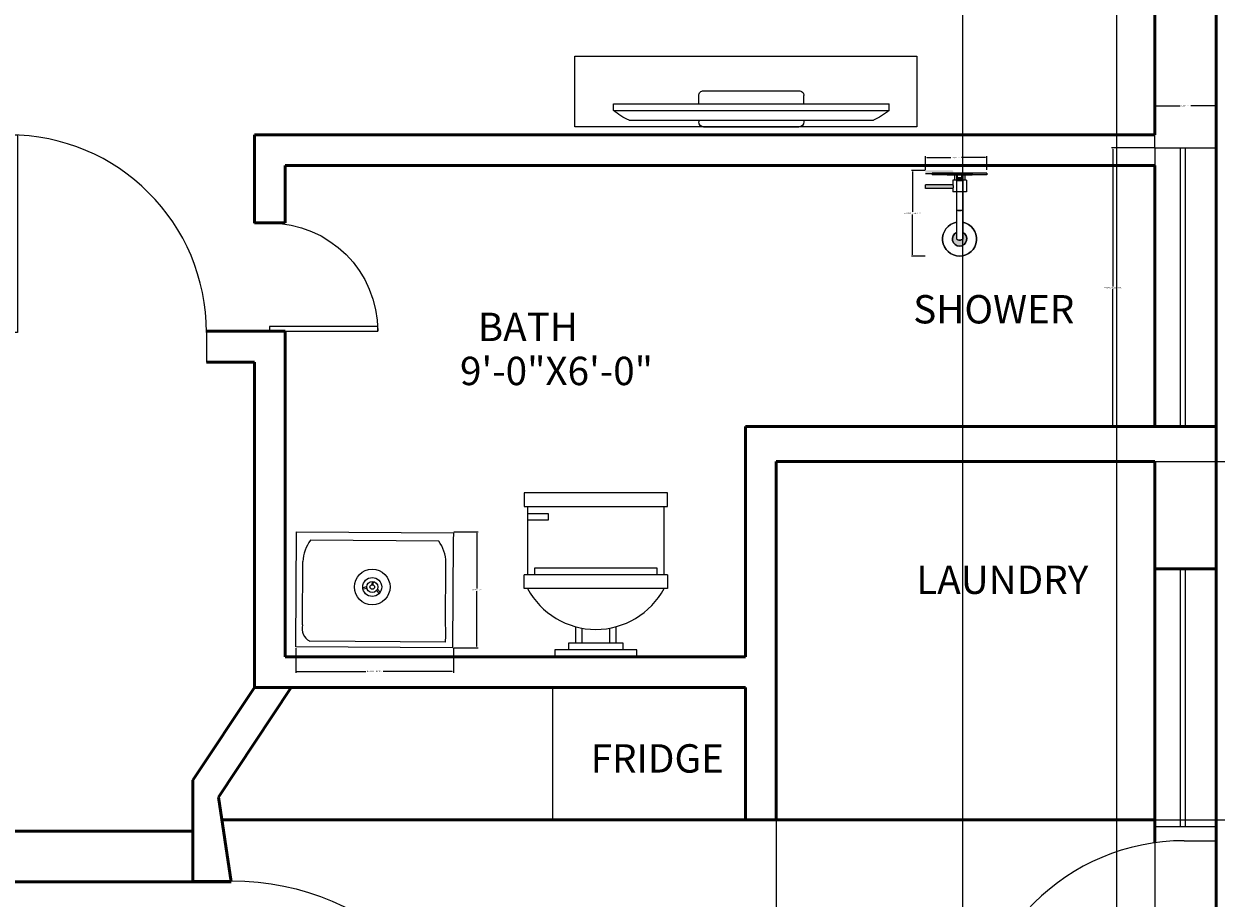
# Model space of a CAD drawing. Units: inches. Extents: x -44 to 461, y -6 to 860.
# Tile 5 of 7: x 184 to 358, y 498 to 626. Entities that reach past the tile are written whole.
import ezdxf

# ---------------------------------------------------------------- set-up
doc = ezdxf.new("R2010")
doc.units = ezdxf.units.IN
doc.header["$MEASUREMENT"] = 0
for name, color, linetype, lineweight in [('A-ANNO-DIMS', 2, 'Continuous', 18), ('A-ANNO-TEXT', 7, 'Continuous', 18), ('A-AREA-IDEN', 7, 'Continuous', 18), ('A-DOOR', 4, 'Continuous', 25), ('A-EQPM', 8, 'Continuous', 18), ('furniture', 30, 'Continuous', 18), ('PLUMBING FIXTURES', 8, 'Continuous', 18), ('walls', 8, 'Continuous', 50), ('windows', 171, 'Continuous', 18)]:
    doc.layers.add(name, color=color, linetype=linetype, lineweight=lineweight)
doc.styles.get("Standard").update_dxf_attribs({"font": 'arial.ttf'})
doc.dimstyles.get("Standard").update_dxf_attribs({"dimtxt": 0.18, "dimasz": 0.18, "dimexe": 0.18, "dimexo": 0.0625, "dimgap": 0.09, "dimtad": 0, "dimtih": 1, "dimtoh": 1, "dimdec": 4, "dimzin": 0, "dimdsep": 46, "dimtxsty": 'Standard', "dimcen": 0.09, "dimadec": 0, "dimazin": 0, "dimtfac": 1, "dimtdec": 4, "dimtofl": 0, "dimtmove": 0, "dimatfit": 3, "dimfxl": 1, "dimtolj": 1, "dimtzin": 0, "dimarcsym": 0})

# ---------------------------------------------------------------- blocks, each defined once
blk = doc.blocks.new('PLASMA-LARGE')
at = {"layer": 'furniture'}
for p, q in [((-7.26, 0), (7.26, 0)), ((-18.61, -1), (18.61, -1)), ((-8, -1), (-8, -0.74)), ((8, -1), (8, -0.74)), ((-21, -2.5), (21, -2.5)), ((-21, -2.5), (-21, -3.5)), ((-21, -3.5), (21, -3.5)), ((-8, -3.5), (-8, -4.76)), ((8, -3.5), (8, -4.76)), ((21, -2.5), (21, -3.5)), ((-7.26, -5.5), (7.26, -5.5))]:
    blk.add_line(p, q, dxfattribs=at)
for centre, radius, start, end in [((-7.26, -0.74), 0.744, 90, 180), ((7.26, -0.74), 0.744, 0, 90), ((-13.97, -11.05), 11.07, 114.7602, 129.4175), ((13.97, -11.05), 11.07, 50.5825, 65.2398), ((-7.26, -4.76), 0.744, 180, 270), ((7.26, -4.76), 0.744, 270, 0)]:
    blk.add_arc(centre, radius, start, end, dxfattribs=at)
blk = doc.blocks.new('*U10')
for p, q in [((-10, 22), (-10, 12)), ((-10, 21), (-7, 21)), ((-7, 21), (-7, 20)), ((10, 12), (10, 22)), ((-7, 20), (-10, 20)), ((9, 13), (-9, 13)), ((-9, 13), (-9, 12)), ((9, 12), (9, 13)), ((10.5, 12), (-10.5, 12)), ((-10.5, 10), (-10.5, 12)), ((10.5, 12), (10.5, 10)), ((10.5, 10), (-10.5, 10)), ((-3, 4.4065), (-3, 2)), ((-2, 2), (-2, 4.1658)), ((2, 4.1658), (2, 2)), ((3, 2), (3, 4.4065)), ((4, 2), (-4, 2)), ((-4, 2), (-4, 1)), ((4, 1), (4, 2))]:
    blk.add_line(p, q)
for points in [[(10.5, 22), (10.5, 24), (-10.5, 24), (-10.5, 22)], [(6, 0), (6, 1), (-6, 1), (-6, 0)]]:
    blk.add_lwpolyline(points, close=True)
blk.add_arc((0, 15.3333), 11.3333, 208.0725, 331.9275)
blk = doc.blocks.new('*U12')
for p, q in [((0, 0), (0, -6)), ((40, 0), (40, -6))]:
    blk.add_line(p, q)
blk.add_lwpolyline([(0, 0), (0, 40), (1.75, 40), (1.75, 0)], close=True)
blk.add_arc((0, 0), 40, 0, 90)
blk = doc.blocks.new('WIN-41IN-FRAME')
for p, q in [((0, 40.98), (9, 40.98)), ((0, 40.98), (0, 0)), ((3.73, 40.98), (3.73, 0)), ((4.5, 0), (4.5, 40.98)), ((9, 40.98), (9, 0)), ((9, 0), (0, 0))]:
    blk.add_line(p, q)
blk = doc.blocks.new('LAV-RECTANGULAR')
for p, q in [((0, 0.15), (0.11, 17)), ((0.11, 17), (23.11, 16.85)), ((20.97, 15.65), (2.16, 15.77)), ((23.11, 16.85), (23.1, 15.71)), ((23.1, 15.71), (23, 0)), ((0.99, 3.35), (1.05, 12.64)), ((21.97, 3.21), (22.03, 12.5)), ((10.4, 8.91), (9.84, 8.81)), ((11.22, 9.73), (11.17, 9.24)), ((11.36, 9.22), (11.4, 9.7)), ((10.52, 8.7), (9.87, 8.58)), ((11.84, 8.39), (12.22, 7.95)), ((11.97, 8.6), (12.36, 8.13)), ((23, 0), (0, 0.15)), ((21.95, 0.84), (2.06, 0.97))]:
    blk.add_line(p, q)
for radius in [2.61, 1.39, 0.816, 0.338]:
    blk.add_circle((11.22, 8.91), radius)
for centre, radius, start, end in [((6.46, 12.5), 5.4, 142.7525, 178.5493), ((16.62, 12.43), 5.4, 0.6949, 36.4918), ((3, 2.82), 2.08, 165.2338, 242.9258), ((12.7, 2.09), 9.33, 352.3124, 6.9318)]:
    blk.add_arc(centre, radius, start, end)
blk = doc.blocks.new('O.H SHOWER-PL')
at = {"layer": 'PLUMBING FIXTURES'}
for points in [[(-1.84, 0), (-1.84, -0.25), (1.84, -0.25), (1.84, 0)], [(0.46, -8.72), (0.46, -9.67, -0.422337), (-0.46, -9.67), (-0.46, -8.72, 4.325472)]]:
    blk.add_hatch(color=256, dxfattribs=at).paths.add_polyline_path(points)
for p, q in [((-1.84, 0), (-1.84, -0.25)), ((1.84, 0), (-1.84, 0)), ((1.84, 0), (1.84, -0.25)), ((1.84, -0.25), (-1.84, -0.25)), ((-0.46, -0.25), (-0.46, -9.67)), ((0.46, -0.25), (0.46, -9.67))]:
    blk.add_line(p, q, dxfattribs=at)
for centre, radius, start, end in [((0, -4.48), 1.03, 243.53, 296.47), ((0, -9.67), 2.5, 100.61, 79.39), ((0, -9.67), 1.05, 116.0349, 63.9652), ((0, -9.22), 0.643, 224.2078, 315.7922)]:
    blk.add_arc(centre, radius, start, end, dxfattribs=at)
blk = doc.blocks.new('DIVERTER-PL')
at = {"layer": 'PLUMBING FIXTURES'}
for points in [[(4, 0), (-4, 0), (-4, -0.25), (4, -0.25)], [(0.38, -1.14), (0.38, -0.7), (-0.37, -0.7), (-0.37, -1.14)], [(1, -1.75, 0.30818), (1, -2.25), (5, -2.25), (5, -1.75)]]:
    blk.add_hatch(color=256, dxfattribs=at).paths.add_polyline_path(points)
for p, q in [((-4, 0), (-4, -0.25)), ((-4, 0), (4, 0)), ((4, 0), (4, -0.25)), ((-4, -0.25), (4, -0.25)), ((-4, -0.25), (4, -0.25)), ((-1, -1.05), (-0.37, -1.05)), ((-1, -1.05), (-1, -2.75)), ((-0.75, -0.25), (-0.75, -1.05)), ((-0.37, -0.7), (0.38, -0.7)), ((-0.37, -0.7), (-0.37, -1.14)), ((-0.37, -1.14), (0.38, -1.14)), ((-0.32, -0.7), (-0.32, -0.25)), ((0.32, -0.7), (0.32, -0.25)), ((0.38, -0.7), (0.38, -1.14)), ((0.38, -1.05), (1, -1.05)), ((0.75, -0.25), (0.75, -1.05)), ((1, -1.05), (1, -1.75)), ((-1, -2.75), (1, -2.75)), ((1, -2.25), (1, -2.75))]:
    blk.add_line(p, q, dxfattribs=at)
at = {"layer": 'PLUMBING FIXTURES', "ltscale": 12}
for p, q in [((1, -1.75), (5, -1.75)), ((1, -2.25), (5, -2.25)), ((5, -2.25), (5, -1.75))]:
    blk.add_line(p, q, dxfattribs=at)
at = {"layer": 'PLUMBING FIXTURES'}
blk.add_arc((1.37, -2), 0.444, 145.7435, 214.2565, dxfattribs=at)
blk = doc.blocks.new('A$C7F153053')
at = {"layer": 'PLUMBING FIXTURES', "xscale": -1, "rotation": 270}
for name in ['DIVERTER-PL', 'O.H SHOWER-PL']:
    blk.add_blockref(name, (12.17, 4), dxfattribs=at)
blk = doc.blocks.new('SHOWER-HEAD-AND-DIVERTER')
for points in [[(4, 12.56, -0.30818), (4, 12.06), (0, 12.06), (0, 12.56)], [(4, 12.56, -0.30818), (4, 12.06), (0, 12.06), (0, 12.56)], [(4, 12.56, -0.30818), (4, 12.06), (0, 12.06), (0, 12.56)], [(4, 12.56, -0.30818), (4, 12.06), (0, 12.06), (0, 12.56)], [(4, 12.56, -0.30818), (4, 12.06), (0, 12.06), (0, 12.56)], [(4, 12.56, -0.30818), (4, 12.06), (0, 12.06), (0, 12.56)], [(4, 12.56, -0.30818), (4, 12.06), (0, 12.06), (0, 12.56)], [(4, 12.56, -0.30818), (4, 12.06), (0, 12.06), (0, 12.56)], [(4, 12.56, -0.30818), (4, 12.06), (0, 12.06), (0, 12.56)], [(4, 12.56, -0.30818), (4, 12.06), (0, 12.06), (0, 12.56)], [(4, 12.56, -0.30818), (4, 12.06), (0, 12.06), (0, 12.56)], [(4, 12.56, -0.30818), (4, 12.06), (0, 12.06), (0, 12.56)], [(4, 12.56, -0.30818), (4, 12.06), (0, 12.06), (0, 12.56)], [(4, 12.56, -0.30818), (4, 12.06), (0, 12.06), (0, 12.56)], [(4, 12.56, -0.30818), (4, 12.06), (0, 12.06), (0, 12.56)], [(4, 12.56, -0.30818), (4, 12.06), (0, 12.06), (0, 12.56)], [(4, 12.56, -0.30818), (4, 12.06), (0, 12.06), (0, 12.56)], [(4, 12.56, -0.30818), (4, 12.06), (0, 12.06), (0, 12.56)], [(4, 12.56, -0.30818), (4, 12.06), (0, 12.06), (0, 12.56)], [(4, 12.56, -0.30818), (4, 12.06), (0, 12.06), (0, 12.56)], [(4, 12.56, -0.30818), (4, 12.06), (0, 12.06), (0, 12.56)], [(4, 12.56, -0.30818), (4, 12.06), (0, 12.06), (0, 12.56)], [(4, 12.56, -0.30818), (4, 12.06), (0, 12.06), (0, 12.56)], [(4, 12.56, -0.30818), (4, 12.06), (0, 12.06), (0, 12.56)], [(4, 12.56, -0.30818), (4, 12.06), (0, 12.06), (0, 12.56)], [(4, 12.56, -0.30818), (4, 12.06), (0, 12.06), (0, 12.56)], [(4, 12.56, -0.30818), (4, 12.06), (0, 12.06), (0, 12.56)], [(4, 12.56, -0.30818), (4, 12.06), (0, 12.06), (0, 12.56)], [(4, 12.56, -0.30818), (4, 12.06), (0, 12.06), (0, 12.56)], [(4, 12.56, -0.30818), (4, 12.06), (0, 12.06), (0, 12.56)], [(4, 12.56, -0.30818), (4, 12.06), (0, 12.06), (0, 12.56)], [(4, 12.56, -0.30818), (4, 12.06), (0, 12.06), (0, 12.56)], [(4, 12.56, -0.30818), (4, 12.06), (0, 12.06), (0, 12.56)], [(4, 12.56, -0.30818), (4, 12.06), (0, 12.06), (0, 12.56)], [(4, 12.56, -0.30818), (4, 12.06), (0, 12.06), (0, 12.56)], [(4, 12.56, -0.30818), (4, 12.06), (0, 12.06), (0, 12.56)], [(4.54, 3.44), (4.54, 2.5, 0.422337), (5.46, 2.5), (5.46, 3.44, -4.325472)], [(4.54, 3.44), (4.54, 2.5, 0.422337), (5.46, 2.5), (5.46, 3.44, -4.325472)], [(4.54, 3.44), (4.54, 2.5, 0.422337), (5.46, 2.5), (5.46, 3.44, -4.325472)], [(4.54, 3.44), (4.54, 2.5, 0.422337), (5.46, 2.5), (5.46, 3.44, -4.325472)], [(4.54, 3.44), (4.54, 2.5, 0.422337), (5.46, 2.5), (5.46, 3.44, -4.325472)], [(4.54, 3.44), (4.54, 2.5, 0.422337), (5.46, 2.5), (5.46, 3.44, -4.325472)], [(4.54, 3.44), (4.54, 2.5, 0.422337), (5.46, 2.5), (5.46, 3.44, -4.325472)], [(4.54, 3.44), (4.54, 2.5, 0.422337), (5.46, 2.5), (5.46, 3.44, -4.325472)], [(4.54, 3.44), (4.54, 2.5, 0.422337), (5.46, 2.5), (5.46, 3.44, -4.325472)], [(4.54, 3.44), (4.54, 2.5, 0.422337), (5.46, 2.5), (5.46, 3.44, -4.325472)], [(4.54, 3.44), (4.54, 2.5, 0.422337), (5.46, 2.5), (5.46, 3.44, -4.325472)], [(4.54, 3.44), (4.54, 2.5, 0.422337), (5.46, 2.5), (5.46, 3.44, -4.325472)], [(4.54, 3.44), (4.54, 2.5, 0.422337), (5.46, 2.5), (5.46, 3.44, -4.325472)], [(4.54, 3.44), (4.54, 2.5, 0.422337), (5.46, 2.5), (5.46, 3.44, -4.325472)], [(4.54, 3.44), (4.54, 2.5, 0.422337), (5.46, 2.5), (5.46, 3.44, -4.325472)], [(4.54, 3.44), (4.54, 2.5, 0.422337), (5.46, 2.5), (5.46, 3.44, -4.325472)], [(4.54, 3.44), (4.54, 2.5, 0.422337), (5.46, 2.5), (5.46, 3.44, -4.325472)], [(4.54, 3.44), (4.54, 2.5, 0.422337), (5.46, 2.5), (5.46, 3.44, -4.325472)], [(4.54, 3.44), (4.54, 2.5, 0.422337), (5.46, 2.5), (5.46, 3.44, -4.325472)], [(4.54, 3.44), (4.54, 2.5, 0.422337), (5.46, 2.5), (5.46, 3.44, -4.325472)], [(4.54, 3.44), (4.54, 2.5, 0.422337), (5.46, 2.5), (5.46, 3.44, -4.325472)], [(4.54, 3.44), (4.54, 2.5, 0.422337), (5.46, 2.5), (5.46, 3.44, -4.325472)], [(4.54, 3.44), (4.54, 2.5, 0.422337), (5.46, 2.5), (5.46, 3.44, -4.325472)], [(4.54, 3.44), (4.54, 2.5, 0.422337), (5.46, 2.5), (5.46, 3.44, -4.325472)], [(4.54, 3.44), (4.54, 2.5, 0.422337), (5.46, 2.5), (5.46, 3.44, -4.325472)], [(4.54, 3.44), (4.54, 2.5, 0.422337), (5.46, 2.5), (5.46, 3.44, -4.325472)], [(4.54, 3.44), (4.54, 2.5, 0.422337), (5.46, 2.5), (5.46, 3.44, -4.325472)], [(4.54, 3.44), (4.54, 2.5, 0.422337), (5.46, 2.5), (5.46, 3.44, -4.325472)], [(4.54, 3.44), (4.54, 2.5, 0.422337), (5.46, 2.5), (5.46, 3.44, -4.325472)], [(4.54, 3.44), (4.54, 2.5, 0.422337), (5.46, 2.5), (5.46, 3.44, -4.325472)], [(4.54, 3.44), (4.54, 2.5, 0.422337), (5.46, 2.5), (5.46, 3.44, -4.325472)], [(4.54, 3.44), (4.54, 2.5, 0.422337), (5.46, 2.5), (5.46, 3.44, -4.325472)], [(4.54, 3.44), (4.54, 2.5, 0.422337), (5.46, 2.5), (5.46, 3.44, -4.325472)], [(4.54, 3.44), (4.54, 2.5, 0.422337), (5.46, 2.5), (5.46, 3.44, -4.325472)], [(4.54, 3.44), (4.54, 2.5, 0.422337), (5.46, 2.5), (5.46, 3.44, -4.325472)], [(4.54, 3.44), (4.54, 2.5, 0.422337), (5.46, 2.5), (5.46, 3.44, -4.325472)], [(4.54, 3.44), (4.54, 2.5, 0.422337), (5.46, 2.5), (5.46, 3.44, -4.325472)], [(4.54, 3.44), (4.54, 2.5, 0.422337), (5.46, 2.5), (5.46, 3.44, -4.325472)]]:
    blk.add_hatch(color=256).paths.add_polyline_path(points)
at = {"ltscale": 12}
blk.add_line((4, 12.06), (0, 12.06), dxfattribs=at)
blk.add_line((4, 12.06), (0, 12.06), dxfattribs=at)
blk.add_line((4, 12.06), (0, 12.06), dxfattribs=at)
blk.add_line((4, 12.06), (0, 12.06), dxfattribs=at)
blk.add_line((4, 12.06), (0, 12.06), dxfattribs=at)
blk.add_line((4, 12.06), (0, 12.06), dxfattribs=at)
blk.add_line((4, 12.06), (0, 12.06), dxfattribs=at)
blk.add_line((4, 12.06), (0, 12.06), dxfattribs=at)
blk.add_line((4, 12.06), (0, 12.06), dxfattribs=at)
blk.add_line((4, 12.06), (0, 12.06), dxfattribs=at)
blk.add_line((4, 12.06), (0, 12.06), dxfattribs=at)
blk.add_line((4, 12.06), (0, 12.06), dxfattribs=at)
blk.add_line((4, 12.06), (0, 12.06), dxfattribs=at)
blk.add_line((4, 12.06), (0, 12.06), dxfattribs=at)
blk.add_line((4, 12.06), (0, 12.06), dxfattribs=at)
blk.add_line((4, 12.06), (0, 12.06), dxfattribs=at)
blk.add_line((4, 12.06), (0, 12.06), dxfattribs=at)
blk.add_line((4, 12.06), (0, 12.06), dxfattribs=at)
blk.add_line((4, 12.06), (0, 12.06), dxfattribs=at)
blk.add_line((4, 12.06), (0, 12.06), dxfattribs=at)
blk.add_line((4, 12.06), (0, 12.06), dxfattribs=at)
blk.add_line((4, 12.06), (0, 12.06), dxfattribs=at)
blk.add_line((4, 12.06), (0, 12.06), dxfattribs=at)
blk.add_line((4, 12.06), (0, 12.06), dxfattribs=at)
blk.add_line((4, 12.06), (0, 12.06), dxfattribs=at)
blk.add_line((4, 12.06), (0, 12.06), dxfattribs=at)
blk.add_line((4, 12.06), (0, 12.06), dxfattribs=at)
blk.add_line((4, 12.06), (0, 12.06), dxfattribs=at)
blk.add_line((4, 12.06), (0, 12.06), dxfattribs=at)
blk.add_line((4, 12.06), (0, 12.06), dxfattribs=at)
blk.add_line((4, 12.06), (0, 12.06), dxfattribs=at)
blk.add_line((4, 12.06), (0, 12.06), dxfattribs=at)
blk.add_line((4, 12.06), (0, 12.06), dxfattribs=at)
blk.add_line((4, 12.06), (0, 12.06), dxfattribs=at)
blk.add_line((4, 12.06), (0, 12.06), dxfattribs=at)
blk.add_line((4, 12.06), (0, 12.06), dxfattribs=at)
blk.add_line((4, 12.06), (0, 12.06), dxfattribs=at)
blk.add_line((4, 12.06), (0, 12.06), dxfattribs=at)
for p, q in [((4.54, 11.92), (4.54, 2.5)), ((4.54, 11.92), (4.54, 2.5)), ((4.54, 11.92), (4.54, 2.5)), ((4.54, 11.92), (4.54, 2.5)), ((4.54, 11.92), (4.54, 2.5)), ((4.54, 11.92), (4.54, 2.5)), ((4.54, 11.92), (4.54, 2.5)), ((4.54, 11.92), (4.54, 2.5)), ((4.54, 11.92), (4.54, 2.5)), ((4.54, 11.92), (4.54, 2.5)), ((4.54, 11.92), (4.54, 2.5)), ((4.54, 11.92), (4.54, 2.5)), ((4.54, 11.92), (4.54, 2.5)), ((4.54, 11.92), (4.54, 2.5)), ((4.54, 11.92), (4.54, 2.5)), ((4.54, 11.92), (4.54, 2.5)), ((4.54, 11.92), (4.54, 2.5)), ((4.54, 11.92), (4.54, 2.5)), ((4.54, 11.92), (4.54, 2.5)), ((4.54, 11.92), (4.54, 2.5)), ((4.54, 11.92), (4.54, 2.5)), ((4.54, 11.92), (4.54, 2.5)), ((4.54, 11.92), (4.54, 2.5)), ((4.54, 11.92), (4.54, 2.5)), ((4.54, 11.92), (4.54, 2.5)), ((4.54, 11.92), (4.54, 2.5)), ((4.54, 11.92), (4.54, 2.5)), ((4.54, 11.92), (4.54, 2.5)), ((4.54, 11.92), (4.54, 2.5)), ((4.54, 11.92), (4.54, 2.5)), ((4.54, 11.92), (4.54, 2.5)), ((4.54, 11.92), (4.54, 2.5)), ((4.54, 11.92), (4.54, 2.5)), ((4.54, 11.92), (4.54, 2.5)), ((4.54, 11.92), (4.54, 2.5)), ((4.54, 11.92), (4.54, 2.5)), ((4.54, 11.92), (4.54, 2.5)), ((4.54, 11.92), (4.54, 2.5)), ((5.46, 11.92), (5.46, 2.5)), ((5.46, 11.92), (5.46, 2.5)), ((5.46, 11.92), (5.46, 2.5)), ((5.46, 11.92), (5.46, 2.5)), ((5.46, 11.92), (5.46, 2.5)), ((5.46, 11.92), (5.46, 2.5)), ((5.46, 11.92), (5.46, 2.5)), ((5.46, 11.92), (5.46, 2.5)), ((5.46, 11.92), (5.46, 2.5)), ((5.46, 11.92), (5.46, 2.5)), ((5.46, 11.92), (5.46, 2.5)), ((5.46, 11.92), (5.46, 2.5)), ((5.46, 11.92), (5.46, 2.5)), ((5.46, 11.92), (5.46, 2.5)), ((5.46, 11.92), (5.46, 2.5)), ((5.46, 11.92), (5.46, 2.5)), ((5.46, 11.92), (5.46, 2.5)), ((5.46, 11.92), (5.46, 2.5)), ((5.46, 11.92), (5.46, 2.5)), ((5.46, 11.92), (5.46, 2.5)), ((5.46, 11.92), (5.46, 2.5)), ((5.46, 11.92), (5.46, 2.5)), ((5.46, 11.92), (5.46, 2.5)), ((5.46, 11.92), (5.46, 2.5)), ((5.46, 11.92), (5.46, 2.5)), ((5.46, 11.92), (5.46, 2.5)), ((5.46, 11.92), (5.46, 2.5)), ((5.46, 11.92), (5.46, 2.5)), ((5.46, 11.92), (5.46, 2.5)), ((5.46, 11.92), (5.46, 2.5)), ((5.46, 11.92), (5.46, 2.5)), ((5.46, 11.92), (5.46, 2.5)), ((5.46, 11.92), (5.46, 2.5)), ((5.46, 11.92), (5.46, 2.5)), ((5.46, 11.92), (5.46, 2.5)), ((5.46, 11.92), (5.46, 2.5)), ((5.46, 11.92), (5.46, 2.5)), ((5.46, 11.92), (5.46, 2.5))]:
    blk.add_line(p, q)
for centre, radius, start, end in [((5, 7.69), 1.03, 243.53, 296.47), ((5, 7.69), 1.03, 243.53, 296.47), ((5, 7.69), 1.03, 243.53, 296.47), ((5, 7.69), 1.03, 243.53, 296.47), ((5, 7.69), 1.03, 243.53, 296.47), ((5, 7.69), 1.03, 243.53, 296.47), ((5, 7.69), 1.03, 243.53, 296.47), ((5, 7.69), 1.03, 243.53, 296.47), ((5, 7.69), 1.03, 243.53, 296.47), ((5, 7.69), 1.03, 243.53, 296.47), ((5, 7.69), 1.03, 243.53, 296.47), ((5, 7.69), 1.03, 243.53, 296.47), ((5, 7.69), 1.03, 243.53, 296.47), ((5, 7.69), 1.03, 243.53, 296.47), ((5, 7.69), 1.03, 243.53, 296.47), ((5, 7.69), 1.03, 243.53, 296.47), ((5, 7.69), 1.03, 243.53, 296.47), ((5, 7.69), 1.03, 243.53, 296.47), ((5, 7.69), 1.03, 243.53, 296.47), ((5, 7.69), 1.03, 243.53, 296.47), ((5, 7.69), 1.03, 243.53, 296.47), ((5, 7.69), 1.03, 243.53, 296.47), ((5, 7.69), 1.03, 243.53, 296.47), ((5, 7.69), 1.03, 243.53, 296.47), ((5, 7.69), 1.03, 243.53, 296.47), ((5, 7.69), 1.03, 243.53, 296.47), ((5, 7.69), 1.03, 243.53, 296.47), ((5, 7.69), 1.03, 243.53, 296.47), ((5, 7.69), 1.03, 243.53, 296.47), ((5, 7.69), 1.03, 243.53, 296.47), ((5, 7.69), 1.03, 243.53, 296.47), ((5, 7.69), 1.03, 243.53, 296.47), ((5, 7.69), 1.03, 243.53, 296.47), ((5, 7.69), 1.03, 243.53, 296.47), ((5, 7.69), 1.03, 243.53, 296.47), ((5, 7.69), 1.03, 243.53, 296.47), ((5, 7.69), 1.03, 243.53, 296.47), ((5, 7.69), 1.03, 243.53, 296.47), ((5, 2.5), 2.5, 100.61, 79.39), ((5, 2.5), 2.5, 100.61, 79.39), ((5, 2.5), 2.5, 100.61, 79.39), ((5, 2.5), 2.5, 100.61, 79.39), ((5, 2.5), 2.5, 100.61, 79.39), ((5, 2.5), 2.5, 100.61, 79.39), ((5, 2.5), 2.5, 100.61, 79.39), ((5, 2.5), 2.5, 100.61, 79.39), ((5, 2.5), 2.5, 100.61, 79.39), ((5, 2.5), 2.5, 100.61, 79.39), ((5, 2.5), 2.5, 100.61, 79.39), ((5, 2.5), 2.5, 100.61, 79.39), ((5, 2.5), 2.5, 100.61, 79.39), ((5, 2.5), 2.5, 100.61, 79.39), ((5, 2.5), 2.5, 100.61, 79.39), ((5, 2.5), 2.5, 100.61, 79.39), ((5, 2.5), 2.5, 100.61, 79.39), ((5, 2.5), 2.5, 100.61, 79.39), ((5, 2.5), 2.5, 100.61, 79.39), ((5, 2.5), 2.5, 100.61, 79.39), ((5, 2.5), 2.5, 100.61, 79.39), ((5, 2.5), 2.5, 100.61, 79.39), ((5, 2.5), 2.5, 100.61, 79.39), ((5, 2.5), 2.5, 100.61, 79.39), ((5, 2.5), 2.5, 100.61, 79.39), ((5, 2.5), 2.5, 100.61, 79.39), ((5, 2.5), 2.5, 100.61, 79.39), ((5, 2.5), 2.5, 100.61, 79.39), ((5, 2.5), 2.5, 100.61, 79.39), ((5, 2.5), 2.5, 100.61, 79.39), ((5, 2.5), 2.5, 100.61, 79.39), ((5, 2.5), 2.5, 100.61, 79.39), ((5, 2.5), 2.5, 100.61, 79.39), ((5, 2.5), 2.5, 100.61, 79.39), ((5, 2.5), 2.5, 100.61, 79.39), ((5, 2.5), 2.5, 100.61, 79.39), ((5, 2.5), 2.5, 100.61, 79.39), ((5, 2.5), 2.5, 100.61, 79.39), ((5, 2.5), 1.05, 116.0348, 63.9651), ((5, 2.5), 1.05, 116.0348, 63.9651), ((5, 2.5), 1.05, 116.0348, 63.9651), ((5, 2.5), 1.05, 116.0348, 63.9651), ((5, 2.5), 1.05, 116.0348, 63.9651), ((5, 2.5), 1.05, 116.0348, 63.9651), ((5, 2.5), 1.05, 116.0348, 63.9651), ((5, 2.5), 1.05, 116.0348, 63.9651), ((5, 2.5), 1.05, 116.0348, 63.9651), ((5, 2.5), 1.05, 116.0348, 63.9651), ((5, 2.5), 1.05, 116.0348, 63.9651), ((5, 2.5), 1.05, 116.0348, 63.9651), ((5, 2.5), 1.05, 116.0348, 63.9651), ((5, 2.5), 1.05, 116.0348, 63.9651), ((5, 2.5), 1.05, 116.0348, 63.9651), ((5, 2.5), 1.05, 116.0348, 63.9651), ((5, 2.5), 1.05, 116.0348, 63.9651), ((5, 2.5), 1.05, 116.0348, 63.9651), ((5, 2.5), 1.05, 116.0348, 63.9651), ((5, 2.5), 1.05, 116.0348, 63.9651), ((5, 2.5), 1.05, 116.0348, 63.9651), ((5, 2.5), 1.05, 116.0348, 63.9651), ((5, 2.5), 1.05, 116.0348, 63.9651), ((5, 2.5), 1.05, 116.0348, 63.9651), ((5, 2.5), 1.05, 116.0348, 63.9651), ((5, 2.5), 1.05, 116.0348, 63.9651), ((5, 2.5), 1.05, 116.0348, 63.9651), ((5, 2.5), 1.05, 116.0348, 63.9651), ((5, 2.5), 1.05, 116.0348, 63.9651), ((5, 2.5), 1.05, 116.0348, 63.9651), ((5, 2.5), 1.05, 116.0348, 63.9651), ((5, 2.5), 1.05, 116.0348, 63.9651), ((5, 2.5), 1.05, 116.0348, 63.9651), ((5, 2.5), 1.05, 116.0348, 63.9651), ((5, 2.5), 1.05, 116.0348, 63.9651), ((5, 2.5), 1.05, 116.0348, 63.9651), ((5, 2.5), 1.05, 116.0348, 63.9651), ((5, 2.5), 1.05, 116.0348, 63.9651), ((5, 2.95), 0.643, 224.2078, 315.7922), ((5, 2.95), 0.643, 224.2078, 315.7922), ((5, 2.95), 0.643, 224.2078, 315.7922), ((5, 2.95), 0.643, 224.2078, 315.7922), ((5, 2.95), 0.643, 224.2078, 315.7922), ((5, 2.95), 0.643, 224.2078, 315.7922), ((5, 2.95), 0.643, 224.2078, 315.7922), ((5, 2.95), 0.643, 224.2078, 315.7922), ((5, 2.95), 0.643, 224.2078, 315.7922), ((5, 2.95), 0.643, 224.2078, 315.7922), ((5, 2.95), 0.643, 224.2078, 315.7922), ((5, 2.95), 0.643, 224.2078, 315.7922), ((5, 2.95), 0.643, 224.2078, 315.7922), ((5, 2.95), 0.643, 224.2078, 315.7922), ((5, 2.95), 0.643, 224.2078, 315.7922), ((5, 2.95), 0.643, 224.2078, 315.7922), ((5, 2.95), 0.643, 224.2078, 315.7922), ((5, 2.95), 0.643, 224.2078, 315.7922), ((5, 2.95), 0.643, 224.2078, 315.7922), ((5, 2.95), 0.643, 224.2078, 315.7922), ((5, 2.95), 0.643, 224.2078, 315.7922), ((5, 2.95), 0.643, 224.2078, 315.7922), ((5, 2.95), 0.643, 224.2078, 315.7922), ((5, 2.95), 0.643, 224.2078, 315.7922), ((5, 2.95), 0.643, 224.2078, 315.7922), ((5, 2.95), 0.643, 224.2078, 315.7922), ((5, 2.95), 0.643, 224.2078, 315.7922), ((5, 2.95), 0.643, 224.2078, 315.7922), ((5, 2.95), 0.643, 224.2078, 315.7922), ((5, 2.95), 0.643, 224.2078, 315.7922), ((5, 2.95), 0.643, 224.2078, 315.7922), ((5, 2.95), 0.643, 224.2078, 315.7922), ((5, 2.95), 0.643, 224.2078, 315.7922), ((5, 2.95), 0.643, 224.2078, 315.7922), ((5, 2.95), 0.643, 224.2078, 315.7922), ((5, 2.95), 0.643, 224.2078, 315.7922), ((5, 2.95), 0.643, 224.2078, 315.7922), ((5, 2.95), 0.643, 224.2078, 315.7922)]:
    blk.add_arc(centre, radius, start, end)
at = {"ltscale": 35, "rotation": 89.99999999999999}
blk.add_blockref('A$C7F153053', (9, 0), dxfattribs=at)
blk = doc.blocks.new('*D26')
at = {"layer": 'A-ANNO-DIMS', "color": 0, "lineweight": -2, "transparency": 16777216}
for p, q in [((349.38, 608.14), (343.12, 608.14)), ((343.3, 607.96), (343.3, 587.83)), ((343.3, 567.34), (343.3, 587.47)), ((349.38, 567.16), (343.12, 567.16))]:
    blk.add_line(p, q, dxfattribs=at)
at = {"layer": 'A-ANNO-DIMS', "color": 0, "transparency": 16777216}
for points in [[(343.27, 607.96), (343.33, 607.96), (343.3, 608.14)], [(343.27, 567.34), (343.33, 567.34), (343.3, 567.16)]]:
    blk.add_solid(points, dxfattribs=at)
at = {"layer": 'Defpoints', "color": 0, "transparency": 16777216}
for p in [(343.3, 608.14), (349.45, 608.14), (349.45, 567.16)]:
    blk.add_point(p, dxfattribs=at)
at = {"layer": 'A-ANNO-DIMS', "color": 0, "transparency": 16777216, "insert": (343.3, 587.65), "char_height": 0.18, "attachment_point": 5}
blk.add_mtext('\\A1;WINDOW 40.9847 TYP.', dxfattribs=at)
blk = doc.blocks.new('*D27')
at = {"layer": 'A-ANNO-DIMS', "color": 0, "lineweight": -2, "transparency": 16777216}
for p, q in [((349.45, 608.21), (349.45, 614.47)), ((349.63, 614.29), (353.17, 614.29)), ((358.27, 614.29), (354.72, 614.29)), ((358.45, 608.21), (358.45, 614.47))]:
    blk.add_line(p, q, dxfattribs=at)
at = {"layer": 'A-ANNO-DIMS', "color": 0, "transparency": 16777216}
for points in [[(349.63, 614.32), (349.63, 614.26), (349.45, 614.29)], [(358.27, 614.32), (358.27, 614.26), (358.45, 614.29)]]:
    blk.add_solid(points, dxfattribs=at)
at = {"layer": 'Defpoints', "color": 0, "transparency": 16777216}
for p in [(358.45, 614.29), (349.45, 608.14), (358.45, 608.14)]:
    blk.add_point(p, dxfattribs=at)
at = {"layer": 'A-ANNO-DIMS', "color": 0, "transparency": 16777216, "insert": (353.95, 614.29), "char_height": 0.18, "attachment_point": 5}
blk.add_mtext('\\A1;9.0000 TYP.', dxfattribs=at)
blk = doc.blocks.new('*D42')
at = {"layer": 'A-ANNO-DIMS', "color": 0, "lineweight": -2, "transparency": 16777216}
for p, q in [((223.5, 534.8), (223.5, 531.21)), ((246.61, 534.8), (246.61, 531.21)), ((223.68, 531.39), (233.8, 531.39)), ((246.43, 531.39), (236.3, 531.39))]:
    blk.add_line(p, q, dxfattribs=at)
at = {"layer": 'A-ANNO-DIMS', "color": 0, "transparency": 16777216}
for points in [[(223.68, 531.42), (223.68, 531.36), (223.5, 531.39)], [(246.43, 531.42), (246.43, 531.36), (246.61, 531.39)]]:
    blk.add_solid(points, dxfattribs=at)
at = {"layer": 'Defpoints', "color": 0, "transparency": 16777216}
for p in [(223.5, 534.86), (246.61, 534.86), (246.61, 531.39)]:
    blk.add_point(p, dxfattribs=at)
at = {"layer": 'A-ANNO-DIMS', "color": 0, "transparency": 16777216, "insert": (235.05, 531.39), "char_height": 0.18, "attachment_point": 5}
blk.add_mtext('\\A1;BASIN 23.1070 TYP.', dxfattribs=at)
blk = doc.blocks.new('*D43')
at = {"layer": 'A-ANNO-DIMS', "color": 0, "lineweight": -2, "transparency": 16777216}
for p, q in [((246.67, 551.86), (250.25, 551.86)), ((250.07, 551.68), (250.07, 543.54)), ((250.07, 535.04), (250.07, 543.18)), ((246.67, 534.86), (250.25, 534.86))]:
    blk.add_line(p, q, dxfattribs=at)
at = {"layer": 'A-ANNO-DIMS', "color": 0, "transparency": 16777216}
for points in [[(250.04, 551.68), (250.1, 551.68), (250.07, 551.86)], [(250.04, 535.04), (250.1, 535.04), (250.07, 534.86)]]:
    blk.add_solid(points, dxfattribs=at)
at = {"layer": 'Defpoints', "color": 0, "transparency": 16777216}
for p in [(246.61, 551.86), (250.07, 551.86), (246.61, 534.86)]:
    blk.add_point(p, dxfattribs=at)
at = {"layer": 'A-ANNO-DIMS', "color": 0, "transparency": 16777216, "insert": (250.07, 543.36), "char_height": 0.18, "attachment_point": 5}
blk.add_mtext('\\A1;16.9995 TYP.', dxfattribs=at)
blk = doc.blocks.new('*D44')
at = {"layer": 'A-ANNO-DIMS', "color": 0, "lineweight": -2, "transparency": 16777216}
for p, q in [((315.77, 604.84), (313.77, 604.84)), ((313.95, 604.66), (313.95, 598.74)), ((313.95, 592.46), (313.95, 598.38)), ((315.77, 592.28), (313.77, 592.28))]:
    blk.add_line(p, q, dxfattribs=at)
at = {"layer": 'A-ANNO-DIMS', "color": 0, "transparency": 16777216}
for points in [[(313.92, 604.66), (313.98, 604.66), (313.95, 604.84)], [(313.92, 592.46), (313.98, 592.46), (313.95, 592.28)]]:
    blk.add_solid(points, dxfattribs=at)
at = {"layer": 'Defpoints', "color": 0, "transparency": 16777216}
for p in [(313.95, 604.84), (315.83, 604.84), (315.83, 592.28)]:
    blk.add_point(p, dxfattribs=at)
at = {"layer": 'A-ANNO-DIMS', "color": 0, "transparency": 16777216, "insert": (313.95, 598.56), "char_height": 0.18, "attachment_point": 5}
blk.add_mtext('\\A1;SHOWER 12.5604 TYP.', dxfattribs=at)
blk = doc.blocks.new('*D45')
at = {"layer": 'A-ANNO-DIMS', "color": 0, "lineweight": -2, "transparency": 16777216}
for p, q in [((315.83, 604.9), (315.83, 606.9)), ((316.01, 606.72), (319.56, 606.72)), ((324.65, 606.72), (321.1, 606.72)), ((324.83, 604.9), (324.83, 606.9))]:
    blk.add_line(p, q, dxfattribs=at)
at = {"layer": 'A-ANNO-DIMS', "color": 0, "transparency": 16777216}
for points in [[(316.01, 606.75), (316.01, 606.69), (315.83, 606.72)], [(324.65, 606.75), (324.65, 606.69), (324.83, 606.72)]]:
    blk.add_solid(points, dxfattribs=at)
at = {"layer": 'Defpoints', "color": 0, "transparency": 16777216}
for p in [(324.83, 606.72), (315.83, 604.84), (324.83, 604.84)]:
    blk.add_point(p, dxfattribs=at)
at = {"layer": 'A-ANNO-DIMS', "color": 0, "transparency": 16777216, "insert": (320.33, 606.72), "char_height": 0.18, "attachment_point": 5}
blk.add_mtext('\\A1;9.0000 TYP.', dxfattribs=at)
blk = doc.blocks.new('*D50')
at = {"layer": 'A-ANNO-DIMS', "color": 0, "lineweight": -2, "transparency": 16777216}
for p, q in [((293.95, 562.12), (293.95, -5.53)), ((349.45, 562.12), (349.45, -5.53)), ((294.13, -5.35), (321.16, -5.35)), ((349.27, -5.35), (322.23, -5.35))]:
    blk.add_line(p, q, dxfattribs=at)
at = {"layer": 'A-ANNO-DIMS', "color": 0, "transparency": 16777216}
for points in [[(294.13, -5.32), (294.13, -5.38), (293.95, -5.35)], [(349.27, -5.32), (349.27, -5.38), (349.45, -5.35)]]:
    blk.add_solid(points, dxfattribs=at)
at = {"layer": 'Defpoints', "color": 0, "transparency": 16777216}
for p in [(293.95, 562.18), (349.45, 562.18), (349.45, -5.35)]:
    blk.add_point(p, dxfattribs=at)
at = {"layer": 'A-ANNO-DIMS', "color": 0, "transparency": 16777216, "insert": (321.7, -5.35), "char_height": 0.18, "attachment_point": 5}
blk.add_mtext('\\A1;55.5000', dxfattribs=at)
blk = doc.blocks.new('*D51')
at = {"layer": 'A-ANNO-DIMS', "color": 0, "lineweight": -2, "transparency": 16777216}
for p, q in [((349.51, 562.18), (461.03, 562.18)), ((460.85, 562), (460.85, 536.08)), ((460.85, 509.8), (460.85, 535.72)), ((349.51, 509.62), (461.03, 509.62))]:
    blk.add_line(p, q, dxfattribs=at)
at = {"layer": 'A-ANNO-DIMS', "color": 0, "transparency": 16777216}
for points in [[(460.82, 562), (460.88, 562), (460.85, 562.18)], [(460.82, 509.8), (460.88, 509.8), (460.85, 509.62)]]:
    blk.add_solid(points, dxfattribs=at)
at = {"layer": 'Defpoints', "color": 0, "transparency": 16777216}
for p in [(349.45, 562.18), (460.85, 562.18), (349.45, 509.62)]:
    blk.add_point(p, dxfattribs=at)
at = {"layer": 'A-ANNO-DIMS', "color": 0, "transparency": 16777216, "insert": (460.85, 535.9), "char_height": 0.18, "attachment_point": 5}
blk.add_mtext('\\A1;52.5561', dxfattribs=at)
blk = doc.blocks.new('*D53')
at = {"layer": 'A-ANNO-DIMS', "color": 0, "lineweight": -2, "transparency": 16777216}
for p, q in [((321.29, 454.3), (321.29, 859.63)), ((321.47, 859.45), (332.05, 859.45)), ((343.69, 859.45), (333.11, 859.45)), ((343.87, 454.3), (343.87, 859.63))]:
    blk.add_line(p, q, dxfattribs=at)
at = {"layer": 'A-ANNO-DIMS', "color": 0, "transparency": 16777216}
for points in [[(321.47, 859.48), (321.47, 859.42), (321.29, 859.45)], [(343.69, 859.48), (343.69, 859.42), (343.87, 859.45)]]:
    blk.add_solid(points, dxfattribs=at)
at = {"layer": 'Defpoints', "color": 0, "transparency": 16777216}
for p in [(343.87, 859.45), (321.29, 454.23), (343.87, 454.23)]:
    blk.add_point(p, dxfattribs=at)
at = {"layer": 'A-ANNO-DIMS', "color": 0, "transparency": 16777216, "insert": (332.58, 859.45), "char_height": 0.18, "attachment_point": 5}
blk.add_mtext('\\A1;22.5824', dxfattribs=at)

msp = doc.modelspace()

# ---------------------------------------------------------------- linework, layer by layer
at = {"layer": 'A-EQPM'}
for p, q in [((261.16958, 529.0501), (261.16958, 509.62308)), ((289.44568, 529.0501), (261.16958, 529.0501)), ((289.44568, 509.62308), (289.44568, 529.0501)), ((261.16958, 509.62308), (289.44568, 509.62308))]:
    msp.add_line(p, q, dxfattribs=at)
at = {"layer": 'furniture'}
msp.add_lwpolyline([(264.41439, 621.59302), (314.56211, 621.59302), (314.56211, 611.22079), (264.41439, 611.22079)], close=True, dxfattribs=at)
msp.add_lwpolyline([(264.41439, 621.59302), (314.56211, 621.59302), (314.56211, 611.22079), (264.41439, 611.22079)], close=True, dxfattribs=at)
at = {"layer": 'walls'}
for p, q in [((358.44568, 752.5501), (358.44568, 262.0501)), ((349.44568, 743.5501), (349.44568, 610.0501)), ((217.44568, 610.0501), (349.44568, 610.0501)), ((217.44568, 610.0501), (217.44568, 597.14022)), ((221.94568, 605.5501), (349.44568, 605.5501)), ((221.94568, 605.5501), (221.94568, 597.14022)), ((349.44568, 605.5501), (349.44568, 567.3001)), ((217.44568, 597.14022), (221.94568, 597.14022)), ((221.94568, 581.25444), (210.42382, 581.25444)), ((221.94568, 581.25444), (221.94568, 533.5501)), ((221.94568, 576.72943), (221.94568, 581.25444)), ((210.42382, 576.72943), (217.44568, 576.72943)), ((217.44568, 576.72943), (217.44568, 529.0501)), ((289.44568, 567.3001), (289.44568, 533.5501)), ((289.44568, 567.3001), (358.44568, 567.3001)), ((358.44568, 546.41584), (358.44568, 567.3001)), ((293.94568, 562.17916), (293.94568, 529.0501)), ((293.94568, 562.17916), (349.44568, 562.17916)), ((349.44568, 562.17916), (349.44568, 506.27408)), ((349.44568, 562.17916), (349.44568, 546.41584)), ((349.44568, 546.41584), (358.44568, 546.41584)), ((221.94568, 533.5501), (289.44568, 533.5501)), ((217.44568, 529.0501), (208.42435, 515.4748)), ((222.84871, 529.0501), (212.17225, 512.98417)), ((217.44568, 529.0501), (289.44568, 529.0501)), ((289.44568, 509.62308), (289.44568, 529.0501)), ((293.94568, 509.62308), (293.94568, 529.0501)), ((349.44568, 529.0501), (349.44568, 506.27408)), ((208.42435, 515.4748), (208.42435, 500.5501)), ((214.03587, 500.5501), (212.17225, 512.98417)), ((289.44568, 509.62308), (212.67601, 509.62308)), ((289.44568, 509.62308), (293.94568, 509.62308)), ((293.94568, 509.62308), (349.44568, 509.62308)), ((155.94568, 507.99109), (208.42435, 507.99109)), ((155.94568, 500.5501), (208.42435, 500.5501)), ((208.42435, 500.5501), (214.03587, 500.5501))]:
    msp.add_line(p, q, dxfattribs=at)
at = {"layer": 'windows'}
for p, q in [((349.44568, 546.41584), (358.44568, 546.41584)), ((349.44568, 546.41584), (349.44568, 508.60271)), ((353.17263, 546.41584), (353.17263, 508.60271)), ((353.94568, 508.60271), (353.94568, 546.41584)), ((358.44568, 546.41584), (358.44568, 508.60271)), ((358.44568, 508.60271), (349.44568, 508.60271))]:
    msp.add_line(p, q, dxfattribs=at)

# ---------------------------------------------------------------- block references
at = {"layer": 'A-DOOR', "xscale": 0.7244533731370114, "yscale": 0.7244533731370114, "zscale": 0.7244533731370114}
msp.add_blockref('*U12', (181.44568, 581.07615), dxfattribs=at)
at = {"layer": 'A-DOOR'}
for p, xscale, yscale, zscale, rotation in [((219.63557, 581.25444), -0.3973109503495726, 0.3973109503495726, 0.3973109503495726, 270), ((353.77957, 475.47002), 0.7776860473082563, 0.7776860473082563, 0.7776860473082563, 90), ((214.10795, 462.80268), -0.9472671488816434, 0.9472671488816434, 0.9472671488816434, 270)]:
    msp.add_blockref('*U12', p, dxfattribs=dict(at, xscale=xscale, yscale=yscale, zscale=zscale, rotation=rotation))
at = {"layer": 'A-EQPM', "xscale": -0.9628364592350681, "yscale": 0.9628364592350692, "zscale": 0.9628364592350692, "rotation": 180.0045102986114}
msp.add_blockref('PLASMA-LARGE', (290.28898, 611.22079), dxfattribs=at)
msp.add_blockref('PLASMA-LARGE', (290.28898, 611.22079), dxfattribs=at)
at = {"layer": 'PLUMBING FIXTURES'}
for name, p in [('SHOWER-HEAD-AND-DIVERTER', (315.8301, 592.279)), ('*U10', (267.49579, 533.5501)), ('LAV-RECTANGULAR', (223.49878, 534.85985))]:
    msp.add_blockref(name, p, dxfattribs=at)
at = {"layer": 'windows'}
msp.add_blockref('WIN-41IN-FRAME', (349.446, 567.15779), dxfattribs=at)

# ---------------------------------------------------------------- texts
at = {"layer": 'A-ANNO-TEXT'}
msp.add_text('FRIDGE', height=4.155577, dxfattribs=at).set_placement((266.74169, 516.56279))
at = {"layer": 'A-AREA-IDEN'}
for s, height, p in [('SHOWER', 4.155577, (314.03117, 582.40234)), ('BATH', 4.155577, (250.18636, 579.81739)), ('9\'-0"X6\'-0"', 4.1555773, (247.58631, 573.35951)), ('LAUNDRY', 4.155577, (314.4785, 542.75739))]:
    msp.add_text(s, height=height, dxfattribs=at).set_placement(p)

# ---------------------------------------------------------------- dimensions: what is measured, and where the dimension line sits
at = {"layer": 'A-ANNO-DIMS'}
for base, p1, p2, picture, middle in [((343.87134, 859.4501), (321.28892, 454.23298), (343.87134, 454.23298), '*D53', (332.58013, 859.4501)), ((349.44569, -5.3499), (293.94569, 562.17916), (349.44569, 562.17916), '*D50', (321.69569, -5.3499))]:
    dim = msp.add_linear_dim(base=base, p1=p1, p2=p2, dimstyle='Standard', override={"dimdec": 4, "dimlfac": 1, "dimrnd": 0, "dimzin": 0, "dimdsep": 46, "dimlunit": 2}, dxfattribs=at)
    dim.commit()
    dim.dimension.update_dxf_attribs({"geometry": picture, "text_midpoint": middle})
for base, p1, p2, text, picture, middle in [((358.44568, 614.29033), (349.44568, 608.14262), (358.44568, 608.14262), '<> TYP.', '*D27', (353.94568, 614.29033)), ((324.82995, 606.72395), (315.82995, 604.83989), (324.82995, 604.83989), '<> TYP.', '*D45', (320.32995, 606.72395)), ((246.60627, 531.39407), (223.49928, 534.86012), (246.60627, 534.86012), 'BASIN <> TYP.', '*D42', (235.05278, 531.39407))]:
    dim = msp.add_linear_dim(base=base, p1=p1, p2=p2, text=text, dimstyle='Standard', override={"dimdec": 4, "dimlfac": 1, "dimrnd": 0, "dimzin": 0, "dimdsep": 46, "dimlunit": 2}, dxfattribs=at)
    dim.commit()
    dim.dimension.update_dxf_attribs({"geometry": picture, "text_midpoint": middle})
for base, p1, p2, text, picture, middle in [((343.29798, 608.14262), (349.44568, 567.1579), (349.44568, 608.14262), 'WINDOW <> TYP.', '*D26', (343.29798, 587.65026)), ((313.94589, 604.83989), (315.82995, 592.27948), (315.82995, 604.83989), 'SHOWER <> TYP.', '*D44', (313.94589, 598.55968)), ((250.07232, 551.85958), (246.60627, 534.86012), (246.60627, 551.85958), '<> TYP.', '*D43', (250.07232, 543.35985))]:
    dim = msp.add_linear_dim(base=base, p1=p1, p2=p2, angle=90, text=text, dimstyle='Standard', override={"dimdec": 4, "dimlfac": 1, "dimrnd": 0, "dimzin": 0, "dimdsep": 46, "dimlunit": 2}, dxfattribs=at)
    dim.commit()
    dim.dimension.update_dxf_attribs({"geometry": picture, "text_midpoint": middle})
dim = msp.add_linear_dim(base=(460.84569, 562.17916), p1=(349.44569, 509.62308), p2=(349.44569, 562.17916), angle=90, dimstyle='Standard', override={"dimdec": 4, "dimlfac": 1, "dimrnd": 0, "dimzin": 0, "dimdsep": 46, "dimlunit": 2}, dxfattribs=at)
dim.commit()
dim.dimension.update_dxf_attribs({"geometry": '*D51', "text_midpoint": (460.84569, 535.90112)})

doc.saveas('drawing.dxf')
